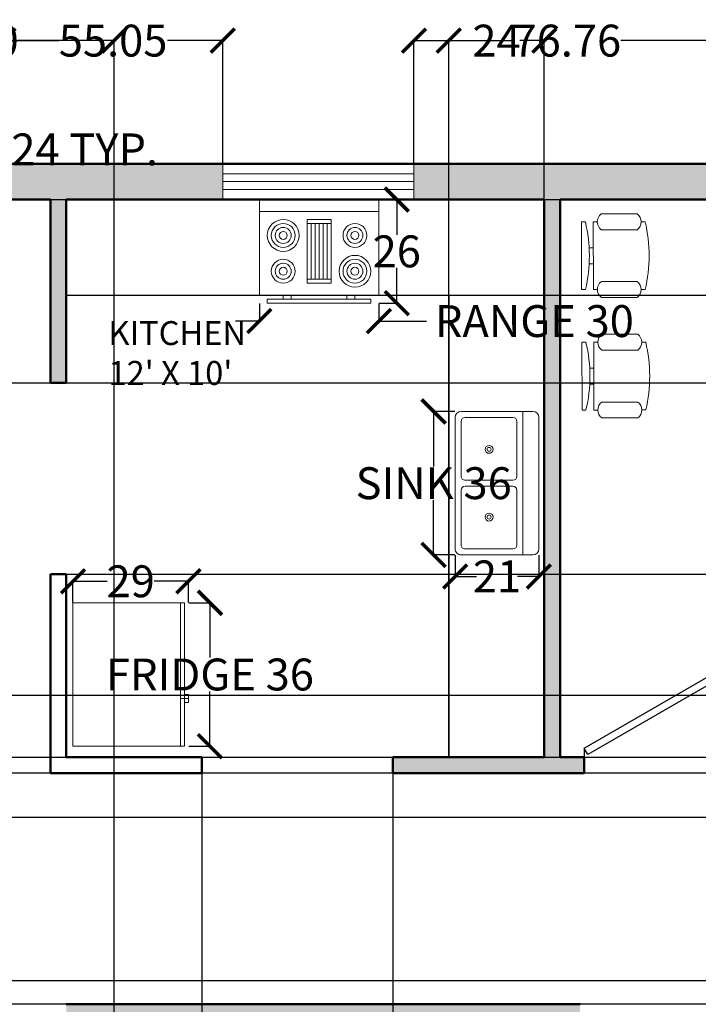
# Model space of a CAD drawing. Units: inches. Extents: x -30 to 744, y -375 to 57.
# Tile 7 of 8: x 355 to 525, y -190 to 57. Entities that reach past the tile are written whole.
import ezdxf

# ---------------------------------------------------------------- set-up
doc = ezdxf.new("R2010")
doc.units = ezdxf.units.IN
doc.header["$MEASUREMENT"] = 0
for name, color, linetype, lineweight in [('A-ANNO-DIMS', 2, 'Continuous', 18), ('A-AREA-IDEN', 7, 'Continuous', 25), ('A-DOOR', 3, 'Continuous', 25), ('A-EQPM', 9, 'Continuous', 18), ('A-FLOR-CASE', 8, 'Continuous', 25), ('A-FLOR-FIXT', 9, 'Continuous', 20), ('A-FURN', 8, 'Continuous', 18), ('A-GLAZ', 4, 'Continuous', 18), ('A-WALL', 7, 'Continuous', 50)]:
    doc.layers.add(name, color=color, linetype=linetype, lineweight=lineweight)
doc.layers.add('A-WALL-PATT', color=251, linetype='Continuous', lineweight=13, true_color=0x636466)
doc.styles.get("Standard").update_dxf_attribs({"font": 'arial.ttf'})
doc.dimstyles.get("Standard").update_dxf_attribs({"dimtxt": 8, "dimasz": 6, "dimexe": 0.18, "dimexo": 0.0625, "dimgap": 0.09, "dimtad": 0, "dimtih": 1, "dimtoh": 1, "dimdec": 0, "dimzin": 0, "dimdsep": 46, "dimlunit": 4, "dimtxsty": 'Standard', "dimblk": 'ARCHTICK', "dimcen": 0.09, "dimadec": 0, "dimazin": 0, "dimtfac": 1, "dimtdec": 0, "dimtofl": 0, "dimtmove": 0, "dimatfit": 1, "dimldrblk": 'ARCHTICK', "dimfxl": 1, "dimtolj": 1, "dimtzin": 0, "dimarcsym": 0})

# ---------------------------------------------------------------- blocks, each defined once
blk = doc.blocks.new('*U2')
for p, q in [((0, 0), (0, -6)), ((40, 0), (40, -6))]:
    blk.add_line(p, q)
blk.add_lwpolyline([(0, 0), (34.64, 20), (35.52, 18.48), (0.87, -1.52)], close=True)
blk.add_arc((0, 0), 40, 0, 30)
blk = doc.blocks.new('Chair - Desk')
for p, q in [((-8.5, 0), (-8.5, -1)), ((-8.5, 0), (8.5, 0)), ((8.5, 0), (8.5, -1)), ((-2, -3), (-2, -1.9355)), ((2, -1.9576), (2, -3)), ((-8.5, -3), (-8.5, -4)), ((-8.5, -3), (8.5, -3)), ((8.5, -3), (8.5, -4)), ((-10.5, -5), (-10.5, -14)), ((-6.5, -14), (-6.5, -5)), ((6.5, -5), (6.5, -14)), ((10.5, -14), (10.5, -5)), ((-8.5, -15), (-8.5, -16)), ((8.5, -15), (8.5, -16))]:
    blk.add_line(p, q)
for centre, radius, start, end in [((0, 34.625), 36.625, 256.5803, 283.4197), ((-8.5, -6.5), 2.5, 36.8699, 143.1301), ((8.5, -6.5), 2.5, 36.8699, 143.1301), ((-8.5, -12.5), 2.5, 216.8699, 323.1301), ((8.5, -12.5), 2.5, 216.8699, 323.1301), ((0, 19.625), 36.625, 256.5803, 283.4197)]:
    blk.add_arc(centre, radius, start, end)
blk = doc.blocks.new('Range-Oven - 30 in top')
for p, q in [((0, -3), (30, -3)), ((12, -6), (18, -6)), ((13, -20), (13, -6)), ((14, -6), (14, -20)), ((15, -20), (15, -6)), ((16, -6), (16, -20)), ((17, -20), (17, -6)), ((18, -20), (12, -20)), ((6, -24), (6, -25)), ((8, -25), (8, -24)), ((22, -25), (22, -24)), ((24, -24), (24, -25))]:
    blk.add_line(p, q)
for points in [[(0, -24), (0, 0), (30, 0), (30, -24)], [(12, -21), (12, -5), (18, -5), (18, -21)], [(2, -26), (2, -25), (28, -25), (28, -26)]]:
    blk.add_lwpolyline(points, close=True)
for centre, radius in [((6, -9), 4), ((6, -9), 3), ((6, -9), 2), ((24, -9), 3), ((24, -9), 2), ((6, -9), 1), ((24, -9), 1), ((24, -18), 4), ((6, -18), 3), ((6, -18), 2), ((6, -18), 1), ((24, -18), 3), ((24, -18), 2), ((24, -18), 1)]:
    blk.add_circle(centre, radius)
blk = doc.blocks.new('Sink-double - 36 in top')
for p, q in [((-18, -4), (18, -4)), ((-0.75, -18.5), (-0.75, -6.5)), ((0.75, -6.5), (0.75, -18.5))]:
    blk.add_line(p, q)
for points in [[(-16.5, 0), (16.5, 0)], [(-18, -19.5), (-18, -1.5)], [(18, -1.5), (18, -19.5)], [(-16.5, -18.5), (-16.5, -6.5)], [(-15.5, -5.5), (-1.75, -5.5)], [(1.75, -5.5), (15.5, -5.5)], [(16.5, -6.5), (16.5, -18.5)], [(-1.75, -19.5), (-15.5, -19.5)], [(15.5, -19.5), (1.75, -19.5)], [(16.5, -21), (-16.5, -21)]]:
    blk.add_lwpolyline(points)
for centre, radius in [((-8.5, -12.5), 1), ((-8.5, -12.5), 0.5), ((8.5, -12.5), 1), ((8.5, -12.5), 0.5)]:
    blk.add_circle(centre, radius)
for centre, radius, start, end in [((-16.5, -1.5), 1.5, 90, 180), ((16.5, -1.5), 1.5, 0, 90), ((-15.5, -6.5), 1, 90, 180), ((-1.75, -6.5), 1, 0, 90), ((1.75, -6.5), 1, 90, 180), ((15.5, -6.5), 1, 0, 90), ((-16.5, -19.5), 1.5, 180, 270), ((-15.5, -18.5), 1, 180, 270), ((-1.75, -18.5), 1, 270, 0), ((1.75, -18.5), 1, 180, 270), ((15.5, -18.5), 1, 270, 0), ((16.5, -19.5), 1.5, 270, 0)]:
    blk.add_arc(centre, radius, start, end)
blk = doc.blocks.new('Refrigerator-2 door - 36 in top')
for p, q in [((0, -26.999999), (36, -26.999999)), ((12, -26.999999), (12, -28.999999)), ((11, -27.999999), (11, -28.999999)), ((11, -28.999999), (13, -28.999999)), ((13, -28.999999), (13, -27.999999))]:
    blk.add_line(p, q)
blk.add_lwpolyline([(0, -27.999999), (0, 0), (36, 0), (36, -27.999999)], close=True)
blk = doc.blocks.new('WIN-48IN')
for p, q in [((0, 0), (0, 48)), ((0, 48), (9, 48)), ((2.5, 48), (2.5, 0)), ((4.5, 48), (4.5, 0)), ((6.5, 48), (6.5, 0)), ((9, 48), (9, 0)), ((9, 48), (9, 0)), ((9, 0), (0, 0))]:
    blk.add_line(p, q)
blk = doc.blocks.new('_ArchTick')
at = {"color": 0, "linetype": 'ByBlock', "const_width": 0.15}
blk.add_lwpolyline([(-0.5, -0.5), (0.5, 0.5)], dxfattribs=at)
blk = doc.blocks.new('*D42')
at = {"layer": 'A-ANNO-DIMS', "color": 0, "lineweight": -2, "transparency": 16777216}
for p, q in [((233.43, 24.3), (227.43, 24.3)), ((233.43, 20.77), (233.43, 24.48)), ((257.43, 20.77), (257.43, 24.48)), ((257.43, 24.3), (269.43, 24.3))]:
    blk.add_line(p, q, dxfattribs=at)
at = {"layer": 'Defpoints', "color": 0, "transparency": 16777216}
for p in [(257.43, 24.3), (233.43, 20.7), (257.43, 20.7)]:
    blk.add_point(p, dxfattribs=at)
at = {"layer": 'A-ANNO-DIMS', "color": 0, "lineweight": -2, "transparency": 16777216, "xscale": 6, "yscale": 6, "zscale": 6}
blk.add_blockref('_ArchTick', (233.43, 24.3), dxfattribs=at)
at = {"layer": 'A-ANNO-DIMS', "color": 0, "lineweight": -2, "transparency": 16777216, "xscale": 6, "yscale": 6, "zscale": 6, "rotation": 180}
blk.add_blockref('_ArchTick', (257.43, 24.3), dxfattribs=at)
at = {"layer": 'A-ANNO-DIMS', "color": 0, "transparency": 16777216, "insert": (331.34, 24.3), "char_height": 8, "attachment_point": 5}
blk.add_mtext('\\A1;BATH WINDOW 24 TYP.', dxfattribs=at)
blk = doc.blocks.new('*D48')
at = {"layer": 'A-ANNO-DIMS', "color": 0, "lineweight": -2, "transparency": 16777216}
for p, q in [((414.7, -14.36), (414.7, -18.98)), ((444.7, -14.36), (444.7, -18.98)), ((414.7, -18.8), (408.7, -18.8)), ((444.7, -18.8), (456.7, -18.8))]:
    blk.add_line(p, q, dxfattribs=at)
at = {"layer": 'Defpoints', "color": 0, "transparency": 16777216}
for p in [(414.7, -14.3), (444.7, -14.3), (444.7, -18.8)]:
    blk.add_point(p, dxfattribs=at)
at = {"layer": 'A-ANNO-DIMS', "color": 0, "lineweight": -2, "transparency": 16777216, "xscale": 6, "yscale": 6, "zscale": 6}
blk.add_blockref('_ArchTick', (414.7, -18.8), dxfattribs=at)
at = {"layer": 'A-ANNO-DIMS', "color": 0, "lineweight": -2, "transparency": 16777216, "xscale": 6, "yscale": 6, "zscale": 6, "rotation": 180}
blk.add_blockref('_ArchTick', (444.7, -18.8), dxfattribs=at)
at = {"layer": 'A-ANNO-DIMS', "color": 0, "transparency": 16777216, "insert": (483.73, -18.8), "char_height": 8, "attachment_point": 5}
blk.add_mtext('\\A1;RANGE 30', dxfattribs=at)
blk = doc.blocks.new('*D49')
at = {"layer": 'A-ANNO-DIMS', "color": 0, "lineweight": -2, "transparency": 16777216}
for p, q in [((444.76, 11.7), (449.38, 11.7)), ((449.2, 11.7), (449.2, 2.88)), ((449.2, -14.3), (449.2, -5.47)), ((444.76, -14.3), (449.38, -14.3))]:
    blk.add_line(p, q, dxfattribs=at)
at = {"layer": 'Defpoints', "color": 0, "transparency": 16777216}
for p in [(444.7, 11.7), (449.2, 11.7), (444.7, -14.3)]:
    blk.add_point(p, dxfattribs=at)
at = {"layer": 'A-ANNO-DIMS', "color": 0, "lineweight": -2, "transparency": 16777216, "xscale": 6, "yscale": 6, "zscale": 6}
for p, rotation in [((449.2, 11.7), 90), ((449.2, -14.3), 270)]:
    blk.add_blockref('_ArchTick', p, dxfattribs=dict(at, rotation=rotation))
at = {"layer": 'A-ANNO-DIMS', "color": 0, "transparency": 16777216, "insert": (449.2, -1.3), "char_height": 8, "attachment_point": 5}
blk.add_mtext('\\A1;26', dxfattribs=at)
blk = doc.blocks.new('*D50')
at = {"layer": 'A-ANNO-DIMS', "color": 0, "lineweight": -2, "transparency": 16777216}
for p, q in [((463.8, -41.49), (458.28, -41.49)), ((458.46, -41.49), (458.46, -55.26)), ((458.46, -77.49), (458.46, -63.72)), ((463.8, -77.49), (458.28, -77.49))]:
    blk.add_line(p, q, dxfattribs=at)
at = {"layer": 'Defpoints', "color": 0, "transparency": 16777216}
for p in [(463.86, -41.49), (458.46, -77.49), (463.86, -77.49)]:
    blk.add_point(p, dxfattribs=at)
at = {"layer": 'A-ANNO-DIMS', "color": 0, "lineweight": -2, "transparency": 16777216, "xscale": 6, "yscale": 6, "zscale": 6}
for p, rotation in [((458.46, -41.49), 90), ((458.46, -77.49), 270)]:
    blk.add_blockref('_ArchTick', p, dxfattribs=dict(at, rotation=rotation))
at = {"layer": 'A-ANNO-DIMS', "color": 0, "transparency": 16777216, "insert": (458.46, -59.49), "char_height": 8, "attachment_point": 5}
blk.add_mtext('\\A1;SINK 36', dxfattribs=at)
blk = doc.blocks.new('*D51')
at = {"layer": 'A-ANNO-DIMS', "color": 0, "lineweight": -2, "transparency": 16777216}
for p, q in [((463.86, -77.56), (463.86, -83.07)), ((484.86, -77.56), (484.86, -83.07)), ((463.86, -82.89), (469.24, -82.89)), ((484.86, -82.89), (479.48, -82.89))]:
    blk.add_line(p, q, dxfattribs=at)
at = {"layer": 'Defpoints', "color": 0, "transparency": 16777216}
for p in [(463.86, -77.49), (484.86, -77.49), (484.86, -82.89)]:
    blk.add_point(p, dxfattribs=at)
at = {"layer": 'A-ANNO-DIMS', "color": 0, "lineweight": -2, "transparency": 16777216, "xscale": 6, "yscale": 6, "zscale": 6, "rotation": 180}
blk.add_blockref('_ArchTick', (463.86, -82.89), dxfattribs=at)
at = {"layer": 'A-ANNO-DIMS', "color": 0, "lineweight": -2, "transparency": 16777216, "xscale": 6, "yscale": 6, "zscale": 6}
blk.add_blockref('_ArchTick', (484.86, -82.89), dxfattribs=at)
at = {"layer": 'A-ANNO-DIMS', "color": 0, "transparency": 16777216, "insert": (474.36, -82.89), "char_height": 8, "attachment_point": 5}
blk.add_mtext('\\A1;21', dxfattribs=at)
blk = doc.blocks.new('*D52')
at = {"layer": 'A-ANNO-DIMS', "color": 0, "lineweight": -2, "transparency": 16777216}
for p, q in [((396.97, -89.51), (402.49, -89.51)), ((402.31, -89.51), (402.31, -103.28)), ((402.31, -125.51), (402.31, -111.74)), ((396.97, -125.51), (402.49, -125.51))]:
    blk.add_line(p, q, dxfattribs=at)
at = {"layer": 'Defpoints', "color": 0, "transparency": 16777216}
for p in [(396.91, -89.51), (402.31, -89.51), (396.91, -125.51)]:
    blk.add_point(p, dxfattribs=at)
at = {"layer": 'A-ANNO-DIMS', "color": 0, "lineweight": -2, "transparency": 16777216, "xscale": 6, "yscale": 6, "zscale": 6}
for p, rotation in [((402.31, -89.51), 90), ((402.31, -125.51), 270)]:
    blk.add_blockref('_ArchTick', p, dxfattribs=dict(at, rotation=rotation))
at = {"layer": 'A-ANNO-DIMS', "color": 0, "transparency": 16777216, "insert": (402.31, -107.51), "char_height": 8, "attachment_point": 5}
blk.add_mtext('\\A1;FRIDGE 36', dxfattribs=at)
blk = doc.blocks.new('*D53')
at = {"layer": 'A-ANNO-DIMS', "color": 0, "lineweight": -2, "transparency": 16777216}
for p, q in [((367.91, -89.45), (367.91, -83.93)), ((396.91, -89.45), (396.91, -83.93)), ((367.91, -84.11), (376.52, -84.11)), ((396.91, -84.11), (388.31, -84.11))]:
    blk.add_line(p, q, dxfattribs=at)
at = {"layer": 'Defpoints', "color": 0, "transparency": 16777216}
for p in [(367.91, -84.11), (367.91, -89.51), (396.91, -89.51)]:
    blk.add_point(p, dxfattribs=at)
at = {"layer": 'A-ANNO-DIMS', "color": 0, "lineweight": -2, "transparency": 16777216, "xscale": 6, "yscale": 6, "zscale": 6, "rotation": 180}
blk.add_blockref('_ArchTick', (367.91, -84.11), dxfattribs=at)
at = {"layer": 'A-ANNO-DIMS', "color": 0, "lineweight": -2, "transparency": 16777216, "xscale": 6, "yscale": 6, "zscale": 6}
blk.add_blockref('_ArchTick', (396.91, -84.11), dxfattribs=at)
at = {"layer": 'A-ANNO-DIMS', "color": 0, "transparency": 16777216, "insert": (382.41, -84.11), "char_height": 8, "attachment_point": 5}
blk.add_mtext('\\A1;29', dxfattribs=at)
blk = doc.blocks.new('*D63')
at = {"layer": 'A-ANNO-DIMS', "color": 0, "lineweight": -2, "transparency": 16777216}
for p, q in [((542.17, -132.3), (-16.61, -132.3)), ((-16.43, -132.3), (-16.43, -157.12)), ((-16.43, -190.3), (-16.43, -165.47)), ((542.17, -190.3), (-16.61, -190.3))]:
    blk.add_line(p, q, dxfattribs=at)
at = {"layer": 'Defpoints', "color": 0, "transparency": 16777216}
for p in [(-16.43, -132.3), (542.24, -132.3), (542.24, -190.3)]:
    blk.add_point(p, dxfattribs=at)
at = {"layer": 'A-ANNO-DIMS', "color": 0, "lineweight": -2, "transparency": 16777216, "xscale": 6, "yscale": 6, "zscale": 6}
for p, rotation in [((-16.43, -132.3), 90), ((-16.43, -190.3), 270)]:
    blk.add_blockref('_ArchTick', p, dxfattribs=dict(at, rotation=rotation))
at = {"layer": 'A-ANNO-DIMS', "color": 0, "transparency": 16777216, "insert": (-16.43, -161.3), "char_height": 8, "attachment_point": 5}
blk.add_mtext('\\A1;58', dxfattribs=at)
blk = doc.blocks.new('*D71')
at = {"layer": 'A-ANNO-DIMS', "color": 0, "lineweight": -2, "transparency": 16777216}
for p, q in [((350.47, 20.77), (350.47, 51.78)), ((350.47, 51.6), (364.37, 51.6)), ((405.51, 51.6), (391.61, 51.6)), ((405.51, 20.77), (405.51, 51.78))]:
    blk.add_line(p, q, dxfattribs=at)
at = {"layer": 'Defpoints', "color": 0, "transparency": 16777216}
for p in [(405.51, 51.6), (350.47, 20.7), (405.51, 20.7)]:
    blk.add_point(p, dxfattribs=at)
at = {"layer": 'A-ANNO-DIMS', "color": 0, "lineweight": -2, "transparency": 16777216, "xscale": 6, "yscale": 6, "zscale": 6, "rotation": 180}
blk.add_blockref('_ArchTick', (350.47, 51.6), dxfattribs=at)
at = {"layer": 'A-ANNO-DIMS', "color": 0, "lineweight": -2, "transparency": 16777216, "xscale": 6, "yscale": 6, "zscale": 6}
blk.add_blockref('_ArchTick', (405.51, 51.6), dxfattribs=at)
at = {"layer": 'A-ANNO-DIMS', "color": 0, "transparency": 16777216, "insert": (377.99, 51.6), "char_height": 8, "attachment_point": 5}
blk.add_mtext('\\A1;55.05', dxfattribs=at)
blk = doc.blocks.new('*D72')
at = {"layer": 'A-ANNO-DIMS', "color": 0, "lineweight": -2, "transparency": 16777216}
for p, q in [((453.51, 20.77), (453.51, 51.78)), ((453.51, 51.6), (478.34, 51.6)), ((530.27, 51.6), (505.45, 51.6)), ((530.27, 20.77), (530.27, 51.78))]:
    blk.add_line(p, q, dxfattribs=at)
at = {"layer": 'Defpoints', "color": 0, "transparency": 16777216}
for p in [(530.27, 51.6), (453.51, 20.7), (530.27, 20.7)]:
    blk.add_point(p, dxfattribs=at)
at = {"layer": 'A-ANNO-DIMS', "color": 0, "lineweight": -2, "transparency": 16777216, "xscale": 6, "yscale": 6, "zscale": 6, "rotation": 180}
blk.add_blockref('_ArchTick', (453.51, 51.6), dxfattribs=at)
at = {"layer": 'A-ANNO-DIMS', "color": 0, "lineweight": -2, "transparency": 16777216, "xscale": 6, "yscale": 6, "zscale": 6}
blk.add_blockref('_ArchTick', (530.27, 51.6), dxfattribs=at)
at = {"layer": 'A-ANNO-DIMS', "color": 0, "transparency": 16777216, "insert": (491.89, 51.6), "char_height": 8, "attachment_point": 5}
blk.add_mtext('\\A1;76.76', dxfattribs=at)
blk = doc.blocks.new('*D74')
at = {"layer": 'A-ANNO-DIMS', "color": 0, "lineweight": -2, "transparency": 16777216}
for p, q in [((318.24, -330.23), (318.24, 51.78)), ((318.24, 51.6), (342.41, 51.6)), ((378.24, 51.6), (354.06, 51.6)), ((378.24, -330.23), (378.24, 51.78))]:
    blk.add_line(p, q, dxfattribs=at)
at = {"layer": 'Defpoints', "color": 0, "transparency": 16777216}
for p in [(378.24, 51.6), (318.24, -330.3), (378.24, -330.3)]:
    blk.add_point(p, dxfattribs=at)
at = {"layer": 'A-ANNO-DIMS', "color": 0, "lineweight": -2, "transparency": 16777216, "xscale": 6, "yscale": 6, "zscale": 6, "rotation": 180}
blk.add_blockref('_ArchTick', (318.24, 51.6), dxfattribs=at)
at = {"layer": 'A-ANNO-DIMS', "color": 0, "lineweight": -2, "transparency": 16777216, "xscale": 6, "yscale": 6, "zscale": 6}
blk.add_blockref('_ArchTick', (378.24, 51.6), dxfattribs=at)
at = {"layer": 'A-ANNO-DIMS', "color": 0, "transparency": 16777216, "insert": (348.24, 51.6), "char_height": 8, "attachment_point": 5}
blk.add_mtext('\\A1;60', dxfattribs=at)
blk = doc.blocks.new('*D75')
at = {"layer": 'A-ANNO-DIMS', "color": 0, "lineweight": -2, "transparency": 16777216}
for p, q in [((40.3, 11.7), (662.32, 11.7)), ((662.14, 11.7), (662.14, -7.12)), ((662.14, -34.3), (662.14, -15.47)), ((40.3, -34.3), (662.32, -34.3))]:
    blk.add_line(p, q, dxfattribs=at)
at = {"layer": 'Defpoints', "color": 0, "transparency": 16777216}
for p in [(40.24, 11.7), (662.14, 11.7), (40.24, -34.3)]:
    blk.add_point(p, dxfattribs=at)
at = {"layer": 'A-ANNO-DIMS', "color": 0, "lineweight": -2, "transparency": 16777216, "xscale": 6, "yscale": 6, "zscale": 6}
for p, rotation in [((662.14, 11.7), 90), ((662.14, -34.3), 270)]:
    blk.add_blockref('_ArchTick', p, dxfattribs=dict(at, rotation=rotation))
at = {"layer": 'A-ANNO-DIMS', "color": 0, "transparency": 16777216, "insert": (662.14, -11.3), "char_height": 8, "attachment_point": 5}
blk.add_mtext('\\A1;46', dxfattribs=at)
blk = doc.blocks.new('*D80')
at = {"layer": 'A-ANNO-DIMS', "color": 0, "lineweight": -2, "transparency": 16777216}
for p, q in [((120.38, -143.3), (662.32, -143.3)), ((662.14, -143.3), (662.14, -159.69)), ((662.14, -184.3), (662.14, -167.9)), ((120.38, -184.3), (662.32, -184.3))]:
    blk.add_line(p, q, dxfattribs=at)
at = {"layer": 'Defpoints', "color": 0, "transparency": 16777216}
for p in [(120.31, -143.3), (662.14, -143.3), (120.31, -184.3)]:
    blk.add_point(p, dxfattribs=at)
at = {"layer": 'A-ANNO-DIMS', "color": 0, "lineweight": -2, "transparency": 16777216, "xscale": 6, "yscale": 6, "zscale": 6}
for p, rotation in [((662.14, -143.3), 90), ((662.14, -184.3), 270)]:
    blk.add_blockref('_ArchTick', p, dxfattribs=dict(at, rotation=rotation))
at = {"layer": 'A-ANNO-DIMS', "color": 0, "transparency": 16777216, "insert": (662.14, -163.8), "char_height": 8, "attachment_point": 5}
blk.add_mtext('\\A1;41', dxfattribs=at)
blk = doc.blocks.new('*D82')
at = {"layer": 'A-ANNO-DIMS', "color": 0, "lineweight": -2, "transparency": 16777216}
for p, q in [((366.3, -34.3), (662.32, -34.3)), ((662.14, -34.3), (662.14, -54.12)), ((662.14, -82.3), (662.14, -62.47)), ((366.3, -82.3), (662.32, -82.3))]:
    blk.add_line(p, q, dxfattribs=at)
at = {"layer": 'Defpoints', "color": 0, "transparency": 16777216}
for p in [(366.24, -34.3), (366.24, -82.3), (662.14, -82.3)]:
    blk.add_point(p, dxfattribs=at)
at = {"layer": 'A-ANNO-DIMS', "color": 0, "lineweight": -2, "transparency": 16777216, "xscale": 6, "yscale": 6, "zscale": 6}
for p, rotation in [((662.14, -34.3), 90), ((662.14, -82.3), 270)]:
    blk.add_blockref('_ArchTick', p, dxfattribs=dict(at, rotation=rotation))
at = {"layer": 'A-ANNO-DIMS', "color": 0, "transparency": 16777216, "insert": (662.14, -58.3), "char_height": 8, "attachment_point": 5}
blk.add_mtext('\\A1;48', dxfattribs=at)
blk = doc.blocks.new('*D83')
at = {"layer": 'A-ANNO-DIMS', "color": 0, "lineweight": -2, "transparency": 16777216}
for p, q in [((400.24, -132.36), (400.24, -370.38)), ((448.24, -132.36), (448.24, -370.38)), ((400.24, -370.2), (418.25, -370.2)), ((448.24, -370.2), (430.22, -370.2))]:
    blk.add_line(p, q, dxfattribs=at)
at = {"layer": 'Defpoints', "color": 0, "transparency": 16777216}
for p in [(400.24, -132.3), (448.24, -132.3), (448.24, -370.2)]:
    blk.add_point(p, dxfattribs=at)
at = {"layer": 'A-ANNO-DIMS', "color": 0, "lineweight": -2, "transparency": 16777216, "xscale": 6, "yscale": 6, "zscale": 6, "rotation": 180}
blk.add_blockref('_ArchTick', (400.24, -370.2), dxfattribs=at)
at = {"layer": 'A-ANNO-DIMS', "color": 0, "lineweight": -2, "transparency": 16777216, "xscale": 6, "yscale": 6, "zscale": 6}
blk.add_blockref('_ArchTick', (448.24, -370.2), dxfattribs=at)
at = {"layer": 'A-ANNO-DIMS', "color": 0, "transparency": 16777216, "insert": (424.24, -370.2), "char_height": 8, "attachment_point": 5}
blk.add_mtext('\\A1;48', dxfattribs=at)
blk = doc.blocks.new('*D84')
at = {"layer": 'A-ANNO-DIMS', "color": 0, "lineweight": -2, "transparency": 16777216}
for p, q in [((366.3, 11.7), (662.32, 11.7)), ((662.14, 11.7), (662.14, 3.81)), ((662.14, -12.3), (662.14, -4.4)), ((366.3, -12.3), (662.32, -12.3))]:
    blk.add_line(p, q, dxfattribs=at)
at = {"layer": 'Defpoints', "color": 0, "transparency": 16777216}
for p in [(366.24, 11.7), (366.24, -12.3), (662.14, -12.3)]:
    blk.add_point(p, dxfattribs=at)
at = {"layer": 'A-ANNO-DIMS', "color": 0, "lineweight": -2, "transparency": 16777216, "xscale": 6, "yscale": 6, "zscale": 6}
for p, rotation in [((662.14, 11.7), 90), ((662.14, -12.3), 270)]:
    blk.add_blockref('_ArchTick', p, dxfattribs=dict(at, rotation=rotation))
at = {"layer": 'A-ANNO-DIMS', "color": 0, "transparency": 16777216, "insert": (662.14, -0.3), "char_height": 8, "attachment_point": 5}
blk.add_mtext('\\A1;24', dxfattribs=at)
blk = doc.blocks.new('*D85')
at = {"layer": 'A-ANNO-DIMS', "color": 0, "lineweight": -2, "transparency": 16777216}
for p, q in [((462.24, -128.23), (462.24, 51.78)), ((462.24, 51.6), (468.36, 51.6)), ((486.24, 51.6), (480.11, 51.6)), ((486.24, -128.23), (486.24, 51.78))]:
    blk.add_line(p, q, dxfattribs=at)
at = {"layer": 'Defpoints', "color": 0, "transparency": 16777216}
for p in [(486.24, 51.6), (462.24, -128.3), (486.24, -128.3)]:
    blk.add_point(p, dxfattribs=at)
at = {"layer": 'A-ANNO-DIMS', "color": 0, "lineweight": -2, "transparency": 16777216, "xscale": 6, "yscale": 6, "zscale": 6, "rotation": 180}
blk.add_blockref('_ArchTick', (462.24, 51.6), dxfattribs=at)
at = {"layer": 'A-ANNO-DIMS', "color": 0, "lineweight": -2, "transparency": 16777216, "xscale": 6, "yscale": 6, "zscale": 6}
blk.add_blockref('_ArchTick', (486.24, 51.6), dxfattribs=at)
at = {"layer": 'A-ANNO-DIMS', "color": 0, "transparency": 16777216, "insert": (474.24, 51.6), "char_height": 8, "attachment_point": 5}
blk.add_mtext('\\A1;24', dxfattribs=at)
blk = doc.blocks.new('*D90')
at = {"layer": 'A-ANNO-DIMS', "color": 0, "lineweight": -2, "transparency": 16777216}
for p, q in [((208.3, -112.68), (662.32, -112.68)), ((662.14, -112.68), (662.14, -116.31)), ((662.14, -128.3), (662.14, -124.66)), ((208.3, -128.3), (662.32, -128.3))]:
    blk.add_line(p, q, dxfattribs=at)
at = {"layer": 'Defpoints', "color": 0, "transparency": 16777216}
for p in [(208.24, -112.68), (208.24, -128.3), (662.14, -128.3)]:
    blk.add_point(p, dxfattribs=at)
at = {"layer": 'A-ANNO-DIMS', "color": 0, "lineweight": -2, "transparency": 16777216, "xscale": 6, "yscale": 6, "zscale": 6}
for p, rotation in [((662.14, -112.68), 90), ((662.14, -128.3), 270)]:
    blk.add_blockref('_ArchTick', p, dxfattribs=dict(at, rotation=rotation))
at = {"layer": 'A-ANNO-DIMS', "color": 0, "transparency": 16777216, "insert": (662.14, -120.49), "char_height": 8, "attachment_point": 5}
blk.add_mtext('\\A1;15.617', dxfattribs=at)

msp = doc.modelspace()

# ---------------------------------------------------------------- hatches: boundary and pattern name
at = {"layer": 'A-WALL-PATT'}
h = msp.add_hatch(color=256, dxfattribs=at)
h.dxf.hatch_style = 1
h.paths.add_polyline_path([(40.2356, 11.7031), (204.2356, 11.7031), (204.2356, -24.2969), (208.2356, -24.2969), (208.2356, 11.7031), (233.4275, 11.7031), (233.4275, 20.7031), (31.2356, 20.7031), (31.2356, -34.2969), (40.2356, -34.2969)])
h.paths.add_polyline_path([(40.2356, -82.2969), (31.2356, -82.2969), (31.2356, -132.2969), (40.2356, -132.2969), (51.0767, -132.2969), (111.3137, -132.2969), (111.3137, -143.2969), (120.3137, -143.2969), (120.3137, -132.2969), (156.2356, -132.2969), (156.2356, -128.2969), (113.6001, -128.2969), (113.6001, -128.3034), (53.6001, -128.3034), (40.2356, -128.2969)])
h.paths.add_polyline_path([(302.4681, 20.7031), (257.4275, 20.7031), (257.4275, 11.7031), (286.2356, 11.7031), (286.2356, -60.2969), (208.2356, -60.2969), (208.2356, -54.2969), (204.2356, -54.2969), (204.2356, -64.2969), (208.2356, -64.2969), (286.2356, -64.2969), (286.2356, -128.2969), (264.8954, -128.2969), (208.2356, -128.2969), (204.2356, -128.2969), (198.2356, -128.2969), (198.2356, -132.2969), (290.2356, -132.2969), (290.2356, -128.2969), (290.2356, 11.7031), (302.4681, 11.7031)])
h.paths.add_polyline_path([(405.515, 20.7031), (350.4681, 20.7031), (350.4681, 11.7031), (362.2356, 11.7031), (362.2356, -34.2969), (366.2356, -34.2969), (366.2356, 11.7031), (405.515, 11.7031)])
h.paths.add_polyline_path([(530.2713, 20.7031), (453.515, 20.7031), (453.515, 11.7031), (486.2356, 11.7031), (486.2356, -128.2969), (448.2356, -128.2969), (448.2356, -132.2969), (486.2356, -132.2969), (490.2356, -132.2969), (496.2356, -132.2969), (496.2356, -128.2969), (490.2356, -128.2969), (490.2356, 11.7031), (530.2713, 11.7031)])
h.paths.add_polyline_path([(631.2356, 20.7031), (578.2713, 20.7031), (578.2713, 11.7031), (622.2356, 11.7031), (622.2356, -37.4001), (631.2356, -37.4001)])
h.paths.add_polyline_path([(631.2356, -85.4001), (622.2356, -85.4001), (622.2356, -91.4001), (622.2356, -103.4001), (622.2356, -128.2969), (538.2356, -128.2969), (538.2356, -132.2969), (538.2356, -154.2969), (542.2356, -154.2969), (542.2356, -132.2969), (575.1375, -132.2969), (585.6313, -131.9348), (585.6438, -132.2969), (622.2356, -132.2969), (622.2356, -147.2969), (631.2356, -147.2969)])
h.paths.add_polyline_path([(631.2356, -171.2969), (622.2356, -171.2969), (622.2356, -185.4028), (622.2356, -186.2969), (622.2356, -190.2969), (542.2356, -190.2969), (542.2356, -184.2969), (538.2356, -184.2969), (538.2356, -190.2969), (538.2356, -194.2969), (622.2356, -194.2969), (622.2356, -237.4632), (631.2356, -237.4632)])
h.paths.add_polyline_path([(631.2356, -285.4632), (622.2356, -285.4632), (622.2356, -330.2969), (490.2356, -330.2969), (490.2356, -194.2969), (494.2356, -194.2969), (495.2356, -194.2969), (495.2356, -190.2969), (494.2356, -190.2969), (490.2356, -190.2969), (486.2356, -190.2969), (366.2356, -190.2969), (366.2356, -194.2969), (486.2356, -194.2969), (486.2356, -330.2969), (426.2356, -330.2969), (426.2356, -339.2969), (631.2356, -339.2969)])
h.paths.add_polyline_path([(378.2356, -330.2969), (318.2356, -330.2969), (318.2356, -194.2969), (324.2356, -194.2969), (324.2356, -190.2969), (318.2356, -190.2969), (314.2356, -190.2969), (314.2356, -194.2969), (314.2356, -330.2969), (278.2356, -330.2969), (278.2356, -339.2969), (378.2356, -339.2969)])
h.paths.add_polyline_path([(190.2356, -330.2969), (40.2356, -330.2969), (40.2356, -318.2969), (31.2356, -318.2969), (31.2356, -330.2969), (31.2356, -339.2969), (190.2356, -339.2969)])
h.paths.add_polyline_path([(230.2356, -330.2969), (194.2356, -330.2969), (194.2356, -194.2969), (194.2356, -190.2969), (190.2356, -190.2969), (184.2356, -190.2969), (184.2356, -194.2969), (190.2356, -194.2969), (190.2356, -339.2969), (230.2356, -339.2969)])
h.paths.add_polyline_path([(142.2356, -190.2969), (120.3137, -190.2969), (120.3137, -184.2969), (116.3137, -184.2969), (111.3137, -184.2969), (111.3137, -190.2969), (40.2356, -190.2969), (31.2356, -190.2969), (31.2356, -194.2969), (31.2356, -206.2969), (40.2356, -206.2969), (40.2356, -194.2969), (142.2356, -194.2969)])

# ---------------------------------------------------------------- linework, layer by layer
at = {"layer": 'A-FLOR-CASE'}
for p, q in [((366.2356, -12.2969), (462.2356, -12.2969)), ((462.2356, -12.2969), (462.2356, -128.2969))]:
    msp.add_line(p, q, dxfattribs=at)
at = {"layer": 'A-WALL'}
for p, q in [((290.2356, 11.7031), (362.2356, 11.7031)), ((362.2356, 11.7031), (362.2356, -34.2969)), ((366.2356, 11.7031), (366.2356, -34.2969)), ((366.2356, 11.7031), (486.2356, 11.7031)), ((486.2356, 11.7031), (486.2356, -128.2969)), ((490.2356, 11.7031), (490.2356, -128.2969)), ((490.2356, 11.7031), (622.2356, 11.7031)), ((362.2356, -34.2969), (366.2356, -34.2969)), ((362.2356, -82.2969), (366.2356, -82.2969)), ((362.2356, -82.2969), (362.2356, -128.2969)), ((366.2356, -82.2969), (366.2356, -128.2969)), ((362.2356, -128.2969), (362.2356, -132.2969)), ((366.2356, -128.2969), (400.2356, -128.2969)), ((400.2356, -132.2969), (400.2356, -128.2969)), ((448.2356, -132.2969), (448.2356, -128.2969)), ((448.2356, -128.2969), (486.2356, -128.2969)), ((490.2356, -128.2969), (496.2356, -128.2969)), ((490.2356, -128.2969), (496.2356, -128.2969)), ((496.2356, -128.2969), (496.2356, -132.2969)), ((362.2356, -132.2969), (400.2356, -132.2969)), ((448.2356, -132.2969), (486.2356, -132.2969)), ((490.2356, -132.2969), (486.2356, -132.2969)), ((490.2356, -132.2969), (496.2356, -132.2969)), ((490.2356, -132.2969), (496.2356, -132.2969)), ((366.2356, -190.2969), (486.2356, -190.2969)), ((486.2356, -190.2969), (490.2356, -190.2969)), ((494.2356, -190.2969), (490.2356, -190.2969)), ((495.2356, -190.2969), (494.2356, -190.2969))]:
    msp.add_line(p, q, dxfattribs=at)
msp.add_lwpolyline([(31.2356, -132.2969), (31.2356, 20.7031), (631.2356, 20.7031), (631.2356, -339.2969), (190.2356, -339.2969)], dxfattribs=at)

# ---------------------------------------------------------------- block references
at = {"layer": 'A-DOOR', "xscale": 1.05, "yscale": 1.05, "zscale": 1.05}
msp.add_blockref('*U2', (496.2356, -125.9969), dxfattribs=at)
at = {"layer": 'A-EQPM'}
msp.add_blockref('Range-Oven - 30 in top', (414.7024, 11.7031), dxfattribs=at)
at = {"layer": 'A-EQPM', "rotation": 90}
msp.add_blockref('Refrigerator-2 door - 36 in top', (367.9119, -125.5107), dxfattribs=at)
at = {"layer": 'A-FLOR-FIXT', "rotation": 270}
msp.add_blockref('Sink-double - 36 in top', (484.8593, -59.4936), dxfattribs=at)
at = {"layer": 'A-FURN', "rotation": 90.0607775495836}
for p in [(495.5446, -2.3987), (495.6896, -32.6263)]:
    msp.add_blockref('Chair - Desk', p, dxfattribs=at)
at = {"layer": 'A-GLAZ', "rotation": 270.0000000000003}
msp.add_blockref('WIN-48IN', (405.5151, 20.7027), dxfattribs=at)

# ---------------------------------------------------------------- texts
at = {"layer": 'A-AREA-IDEN', "insert": (376.8432, -18.8151), "char_height": 6, "attachment_point": 1}
msp.add_mtext_dynamic_manual_height_columns("KITCHEN\\P12' X 10'", width=75.228552, gutter_width=1, heights=[0], dxfattribs=at)

# ---------------------------------------------------------------- dimensions: what is measured, and where the dimension line sits
at = {"layer": 'A-ANNO-DIMS'}
for base, p1, p2, override, picture, middle in [((378.2356, 51.6031), (318.2356, -330.2969), (378.2356, -330.2969), {"dimdec": 0, "dimlfac": 1, "dimrnd": 0, "dimzin": 0, "dimdsep": 46, "dimlunit": 2}, '*D74', (348.2356, 51.6031)), ((405.515, 51.6031), (350.4681, 20.7031), (405.515, 20.7031), {"dimdec": 2, "dimlfac": 1, "dimrnd": 0, "dimzin": 0, "dimdsep": 46, "dimlunit": 2}, '*D71', (377.9915, 51.6031)), ((530.2713, 51.6031), (453.515, 20.7031), (530.2713, 20.7031), {"dimdec": 2, "dimlfac": 1, "dimrnd": 0, "dimzin": 0, "dimdsep": 46, "dimlunit": 2}, '*D72', (491.8931, 51.6031)), ((486.2356, 51.6031), (462.2356, -128.2969), (486.2356, -128.2969), {"dimdec": 0, "dimlfac": 1, "dimrnd": 0, "dimzin": 0, "dimdsep": 46, "dimlunit": 2}, '*D85', (474.2356, 51.6031)), ((484.8593, -82.8936), (463.8593, -77.4936), (484.8593, -77.4936), {"dimdec": 0, "dimlfac": 1, "dimrnd": 0, "dimzin": 0, "dimdsep": 46, "dimlunit": 2}, '*D51', (474.3593, -82.8936)), ((448.2356, -370.1969), (400.2356, -132.2969), (448.2356, -132.2969), {"dimdec": 0, "dimlfac": 1, "dimrnd": 0, "dimzin": 0, "dimdsep": 46, "dimlunit": 2}, '*D83', (424.2356, -370.1969))]:
    dim = msp.add_linear_dim(base=base, p1=p1, p2=p2, dimstyle='Standard', override=override, dxfattribs=at)
    dim.commit()
    dim.dimension.update_dxf_attribs({"geometry": picture, "text_midpoint": middle})
for base, p1, p2, text, picture, middle in [((257.4275, 24.3031), (233.4275, 20.7031), (257.4275, 20.7031), 'BATH WINDOW <> TYP.', '*D42', (331.3374, 24.3031)), ((444.7024, -18.7969), (414.7024, -14.2969), (444.7024, -14.2969), 'RANGE <>', '*D48', (483.7256, -18.7969))]:
    dim = msp.add_linear_dim(base=base, p1=p1, p2=p2, text=text, dimstyle='Standard', override={"dimdec": 0, "dimlfac": 1, "dimrnd": 0, "dimzin": 0, "dimdsep": 46, "dimlunit": 2}, dxfattribs=at)
    dim.commit()
    dim.dimension.update_dxf_attribs({"geometry": picture, "text_midpoint": middle})
for base, p1, p2, angle, override, picture, middle in [((662.1356, 11.7031), (40.2356, -34.2969), (40.2356, 11.7031), 90, {"dimdec": 0, "dimlfac": 1, "dimrnd": 0, "dimzin": 0, "dimdsep": 46, "dimlunit": 2}, '*D75', (662.1356, -11.2969)), ((662.1356, -12.2969), (366.2356, 11.7031), (366.2356, -12.2969), 90, {"dimdec": 0, "dimlfac": 1, "dimrnd": 0, "dimzin": 0, "dimdsep": 46, "dimlunit": 2}, '*D84', (662.1356, -0.2969)), ((449.2024, 11.7031), (444.7024, -14.2969), (444.7024, 11.7031), 90, {"dimdec": 0, "dimlfac": 1, "dimrnd": 0, "dimzin": 0, "dimdsep": 46, "dimlunit": 2}, '*D49', (449.2024, -1.2969)), ((662.1356, -82.2969), (366.2356, -34.2969), (366.2356, -82.2969), 90, {"dimdec": 0, "dimlfac": 1, "dimrnd": 0, "dimzin": 0, "dimdsep": 46, "dimlunit": 2}, '*D82', (662.1356, -58.2969)), ((367.9119, -84.1107), (396.9119, -89.5107), (367.9119, -89.5107), 180, {"dimdec": 0, "dimlfac": 1, "dimrnd": 0, "dimzin": 0, "dimdsep": 46, "dimlunit": 2}, '*D53', (382.4119, -84.1107)), ((662.1356, -128.2969), (208.2356, -112.6796), (208.2356, -128.2969), 90, {"dimdec": 3, "dimlfac": 1, "dimrnd": 0, "dimzin": 0, "dimdsep": 46, "dimlunit": 2}, '*D90', (662.1356, -120.4882)), ((-16.4253, -132.2969), (542.2356, -190.2969), (542.2356, -132.2969), 90, {"dimdec": 0, "dimlfac": 1, "dimrnd": 0, "dimzin": 0, "dimdsep": 46, "dimlunit": 2}, '*D63', (-16.4253, -161.2969)), ((662.1356, -143.2969), (120.3137, -184.2969), (120.3137, -143.2969), 90, {"dimdec": 0, "dimlfac": 1, "dimrnd": 0, "dimzin": 0, "dimdsep": 46, "dimlunit": 2}, '*D80', (662.1356, -163.7969))]:
    dim = msp.add_linear_dim(base=base, p1=p1, p2=p2, angle=angle, dimstyle='Standard', override=override, dxfattribs=at)
    dim.commit()
    dim.dimension.update_dxf_attribs({"geometry": picture, "text_midpoint": middle})
for base, p1, p2, angle, text, picture, middle in [((458.4593, -77.4936), (463.8593, -41.4936), (463.8593, -77.4936), 270, 'SINK <>', '*D50', (458.4593, -59.4936)), ((402.3119, -89.5107), (396.9119, -125.5107), (396.9119, -89.5107), 90, 'FRIDGE <>', '*D52', (402.3119, -107.5107))]:
    dim = msp.add_linear_dim(base=base, p1=p1, p2=p2, angle=angle, text=text, dimstyle='Standard', override={"dimdec": 0, "dimlfac": 1, "dimrnd": 0, "dimzin": 0, "dimdsep": 46, "dimlunit": 2}, dxfattribs=at)
    dim.commit()
    dim.dimension.update_dxf_attribs({"geometry": picture, "text_midpoint": middle})

doc.saveas('drawing.dxf')
